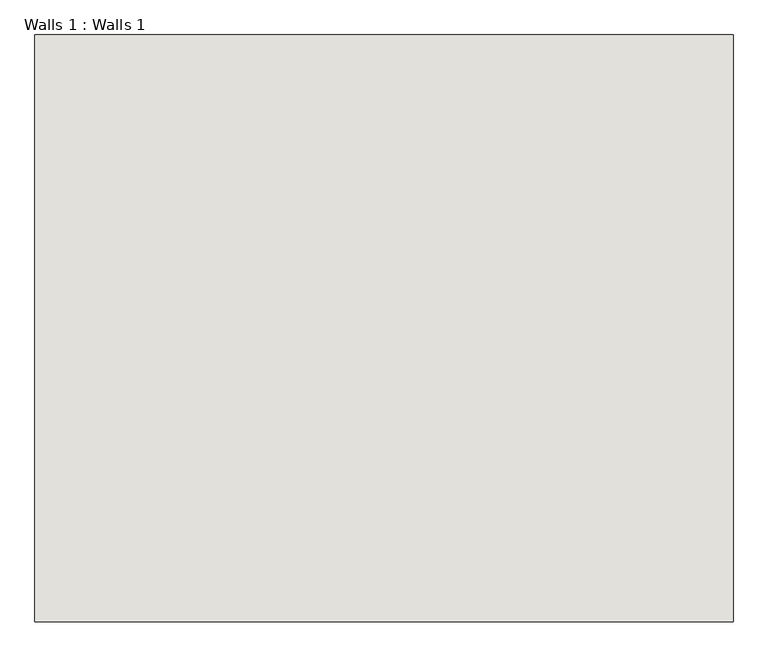
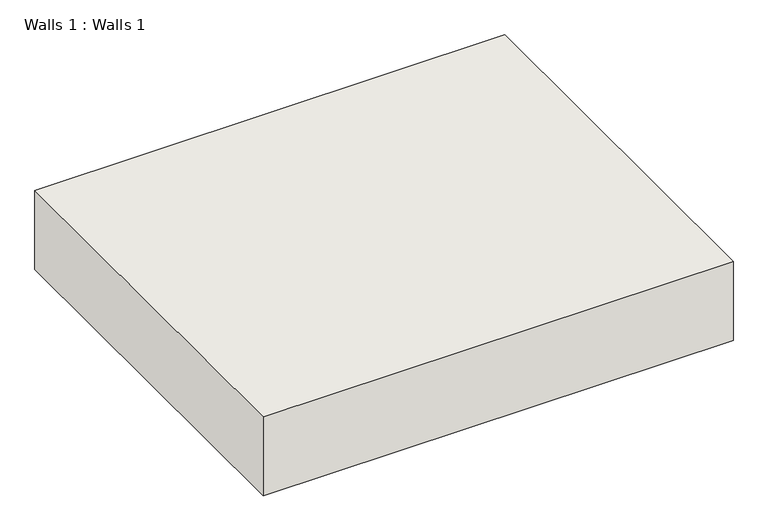
"""IFC4 building model written with IfcOpenShell, lengths in millimetres: wall geometry, Walls 1 : Walls 1."""

from ifc_helpers import new_model, si_unit, frame, origin, place, context, project, spatial, polyline, outline, extrude, source, transform, mapped, element, save


def walls_1_walls_1_cd3f7b89(model_context):
    return source(origin(), model_context, "Body", "SweptSolid", [
        extrude(outline(polyline([(-540.6620963, -5013.5705746), (-4731.6620963, -5013.5705746), (-4731.6620963, -1489.852665), (-540.6620963, -1489.852665), (-540.6620963, -5013.5705746)])), frame((0.0, 0.0, 8194.5880083), z_axis=(0.0, 0.0, 1.0), x_axis=(1.0, 0.0, 0.0)), (0.0, 0.0, 1.0), 746.2119917),
    ])


if __name__ == "__main__":
    model = new_model("IFC4")
    model_context = context("Model", 3, world=origin())
    ifc_project = project(units=[si_unit("LENGTHUNIT", "METRE", prefix="MILLI")], contexts=[model_context])
    site = spatial("IfcSite", under=ifc_project)
    building = spatial("IfcBuilding", under=site)
    placement = place(None, origin())
    walls_1_walls_1_shape = walls_1_walls_1_cd3f7b89(model_context)
    element("IfcWall", 1, ObjectType="Walls 1 : Walls 1", at=placement, inside=building, context=model_context, shape_type="MappedRepresentation", body=[
        mapped(walls_1_walls_1_shape, transform((0.0, 0.0, 0.0), x_axis=(1.0, 0.0, 0.0), y_axis=(0.0, 1.0, 0.0), z_axis=(0.0, 0.0, 1.0))),
    ])
    save(model, "model.ifc")

# Revit data of these elements
# Element 1 (IfcWall, "Walls 1 : Walls 1")
#   Materials on its faces: "Default Wall"
# Materials
#   "Default Wall": colour RGB 128 128 128, transparency 0
